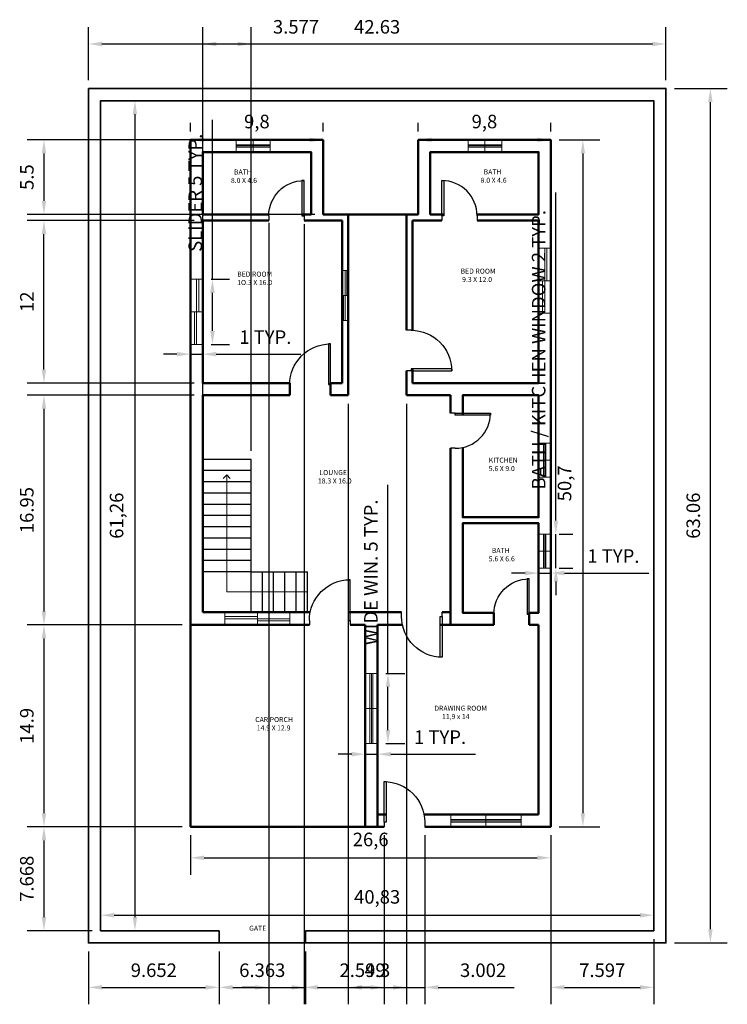
# Model space of a CAD drawing. Units: feet. Extents: x 4235.7 to 4288, y 3917.3 to 3989.9.
import ezdxf

# ---------------------------------------------------------------- set-up
doc = ezdxf.new("R2010")
doc.units = ezdxf.units.FT
for name, color, linetype, lineweight in [('A-ANNO-DIMS', 5, 'Continuous', 18), ('A-ANNO-SYMB', 240, 'Continuous', 18), ('A-ANNO-TEXT', 3, 'Continuous', 30), ('A-AREA-IDEN', 3, 'Continuous', 30), ('A-DOOR', 5, 'Continuous', 25), ('A-FLOR-STRS', 7, 'Continuous', 25), ('A-GLAZ', 2, 'Continuous', 18), ('A-WALL', 7, 'Continuous', 50), ('C-PROP', 242, 'Continuous', 35)]:
    doc.layers.add(name, color=color, linetype=linetype, lineweight=lineweight)
doc.styles.get("Standard").update_dxf_attribs({"font": 'arial.ttf'})
doc.dimstyles.new('ISO-25', dxfattribs={"dimtxt": 1, "dimasz": 1, "dimexe": 1.25, "dimexo": 0.625, "dimtad": 1, "dimtxsty": 'Standard', "dimcen": 1, "dimadec": 0, "dimazin": 0, "dimtfac": 1, "dimtmove": 0, "dimatfit": 3, "dimfxl": 1, "dimarcsym": 0})

# ---------------------------------------------------------------- blocks, each defined once
blk = doc.blocks.new('*U2')
for p, q in [((0, 0), (0, -100)), ((900, 0), (900, -100))]:
    blk.add_line(p, q)
blk.add_lwpolyline([(0, 0), (0, 900), (43.75, 900), (43.75, 0)], close=True)
blk.add_arc((0, 0), 900, 0, 90)
blk = doc.blocks.new('*U3')
for p, q in [((0, 0), (0, -100)), ((750, 0), (750, -100))]:
    blk.add_line(p, q)
blk.add_lwpolyline([(0, 0), (0, 750), (43.75, 750), (43.75, 0)], close=True)
blk.add_arc((0, 0), 750, 0, 90)
blk = doc.blocks.new('*U4')
for p, q in [((0, 0), (0, 100)), ((900, 0), (900, 100))]:
    blk.add_line(p, q)
blk.add_lwpolyline([(0, 0), (0, -900), (43.75, -900), (43.75, 0)], close=True)
blk.add_arc((0, 0), 900, 270, 0)
blk = doc.blocks.new('*U5')
for p, q in [((0, 0), (0, -100)), ((-900, 0), (-900, -100))]:
    blk.add_line(p, q)
blk.add_lwpolyline([(0, 0), (0, 900), (-43.75, 900), (-43.75, 0)], close=True)
blk.add_arc((0, 0), 900, 90, 180)
blk = doc.blocks.new('*D6')
at = {"layer": 'A-ANNO-DIMS', "color": 0, "lineweight": -2, "transparency": 16777216}
for p, q in [((4275.582, 3981.069), (4278.576, 3981.069)), ((4277.326, 3980.069), (4277.326, 3931.369)), ((4275.582, 3930.369), (4278.576, 3930.369))]:
    blk.add_line(p, q, dxfattribs=at)
at = {"layer": 'A-ANNO-DIMS', "color": 0, "transparency": 16777216}
for points in [[(4277.159, 3980.069), (4277.493, 3980.069), (4277.326, 3981.069)], [(4277.159, 3931.369), (4277.493, 3931.369), (4277.326, 3930.369)]]:
    blk.add_solid(points, dxfattribs=at)
at = {"layer": 'Defpoints', "color": 0, "transparency": 16777216}
for p in [(4274.957, 3981.069), (4274.957, 3930.369), (4277.326, 3930.369)]:
    blk.add_point(p, dxfattribs=at)
at = {"layer": 'A-ANNO-DIMS', "color": 0, "transparency": 16777216, "insert": (4276.1, 3955.719), "char_height": 1, "attachment_point": 5, "rotation": 90}
blk.add_mtext('50,7', dxfattribs=at)
blk = doc.blocks.new('*D7')
at = {"layer": 'A-ANNO-DIMS', "color": 0, "lineweight": -2, "transparency": 16777216}
for p, q in [((4248.357, 3981.694), (4248.357, 3982.319)), ((4258.157, 3981.694), (4258.157, 3982.319)), ((4249.357, 3981.069), (4257.157, 3981.069))]:
    blk.add_line(p, q, dxfattribs=at)
at = {"layer": 'A-ANNO-DIMS', "color": 0, "transparency": 16777216}
for points in [[(4249.357, 3981.236), (4249.357, 3980.902), (4248.357, 3981.069)], [(4257.157, 3981.236), (4257.157, 3980.902), (4258.157, 3981.069)]]:
    blk.add_solid(points, dxfattribs=at)
at = {"layer": 'Defpoints', "color": 0, "transparency": 16777216}
for p in [(4248.357, 3981.069), (4258.157, 3981.069), (4258.157, 3981.069)]:
    blk.add_point(p, dxfattribs=at)
at = {"layer": 'A-ANNO-DIMS', "color": 0, "transparency": 16777216, "insert": (4253.257, 3982.295), "char_height": 1, "attachment_point": 5}
blk.add_mtext('9,8', dxfattribs=at)
blk = doc.blocks.new('*D8')
at = {"layer": 'A-ANNO-DIMS', "color": 0, "lineweight": -2, "transparency": 16777216}
for p, q in [((4265.157, 3981.694), (4265.157, 3982.319)), ((4274.957, 3981.694), (4274.957, 3982.319)), ((4266.157, 3981.069), (4273.957, 3981.069))]:
    blk.add_line(p, q, dxfattribs=at)
at = {"layer": 'A-ANNO-DIMS', "color": 0, "transparency": 16777216}
for points in [[(4266.157, 3981.236), (4266.157, 3980.902), (4265.157, 3981.069)], [(4273.957, 3981.236), (4273.957, 3980.902), (4274.957, 3981.069)]]:
    blk.add_solid(points, dxfattribs=at)
at = {"layer": 'Defpoints', "color": 0, "transparency": 16777216}
for p in [(4265.157, 3981.069), (4274.957, 3981.069), (4274.957, 3981.069)]:
    blk.add_point(p, dxfattribs=at)
at = {"layer": 'A-ANNO-DIMS', "color": 0, "transparency": 16777216, "insert": (4270.057, 3982.295), "char_height": 1, "attachment_point": 5}
blk.add_mtext('9,8', dxfattribs=at)
blk = doc.blocks.new('*D9')
at = {"layer": 'A-ANNO-DIMS', "color": 0, "lineweight": -2, "transparency": 16777216}
for p, q in [((4248.357, 3929.744), (4248.357, 3926.829)), ((4274.957, 3929.744), (4274.957, 3926.829)), ((4249.357, 3928.079), (4273.957, 3928.079))]:
    blk.add_line(p, q, dxfattribs=at)
at = {"layer": 'A-ANNO-DIMS', "color": 0, "transparency": 16777216}
for points in [[(4249.357, 3928.245), (4249.357, 3927.912), (4248.357, 3928.079)], [(4273.957, 3928.245), (4273.957, 3927.912), (4274.957, 3928.079)]]:
    blk.add_solid(points, dxfattribs=at)
at = {"layer": 'Defpoints', "color": 0, "transparency": 16777216}
for p in [(4248.357, 3930.369), (4274.957, 3930.369), (4274.957, 3928.079)]:
    blk.add_point(p, dxfattribs=at)
at = {"layer": 'A-ANNO-DIMS', "color": 0, "transparency": 16777216, "insert": (4261.657, 3929.305), "char_height": 1, "attachment_point": 5}
blk.add_mtext('26,6', dxfattribs=at)
blk = doc.blocks.new('*D10')
at = {"layer": 'A-ANNO-DIMS', "color": 0, "lineweight": -2, "transparency": 16777216}
for p, q in [((4241.721, 3923.326), (4241.721, 3925.09)), ((4282.554, 3923.326), (4282.554, 3925.09)), ((4242.721, 3923.84), (4281.554, 3923.84))]:
    blk.add_line(p, q, dxfattribs=at)
at = {"layer": 'A-ANNO-DIMS', "color": 0, "transparency": 16777216}
for points in [[(4242.721, 3924.006), (4242.721, 3923.673), (4241.721, 3923.84)], [(4281.554, 3924.006), (4281.554, 3923.673), (4282.554, 3923.84)]]:
    blk.add_solid(points, dxfattribs=at)
at = {"layer": 'Defpoints', "color": 0, "transparency": 16777216}
for p in [(4282.554, 3923.84), (4241.721, 3922.701), (4282.554, 3922.701)]:
    blk.add_point(p, dxfattribs=at)
at = {"layer": 'A-ANNO-DIMS', "color": 0, "transparency": 16777216, "insert": (4262.137, 3925.066), "char_height": 1, "attachment_point": 5}
blk.add_mtext('40,83', dxfattribs=at)
blk = doc.blocks.new('*D11')
at = {"layer": 'A-ANNO-DIMS', "color": 0, "lineweight": -2, "transparency": 16777216}
for p, q in [((4242.346, 3983.964), (4245.502, 3983.964)), ((4244.252, 3982.964), (4244.252, 3923.701)), ((4242.346, 3922.701), (4245.502, 3922.701))]:
    blk.add_line(p, q, dxfattribs=at)
at = {"layer": 'A-ANNO-DIMS', "color": 0, "transparency": 16777216}
for points in [[(4244.085, 3982.964), (4244.418, 3982.964), (4244.252, 3983.964)], [(4244.085, 3923.701), (4244.418, 3923.701), (4244.252, 3922.701)]]:
    blk.add_solid(points, dxfattribs=at)
at = {"layer": 'Defpoints', "color": 0, "transparency": 16777216}
for p in [(4241.721, 3983.964), (4241.721, 3922.701), (4244.252, 3922.701)]:
    blk.add_point(p, dxfattribs=at)
at = {"layer": 'A-ANNO-DIMS', "color": 0, "transparency": 16777216, "insert": (4243.026, 3953.333), "char_height": 1, "attachment_point": 5, "rotation": 90}
blk.add_mtext('61,26', dxfattribs=at)
blk = doc.blocks.new('WIN-2.496FT')
for p, q in [((0, 2.496), (0.9, 2.496)), ((0.37, 2.496), (0.37, 0)), ((0.45, 2.496), (0.45, 0)), ((0.53, 2.496), (0.53, 0)), ((0.9, 1.248), (0, 1.248)), ((0.45, 1.248), (0.9, 1.248)), ((0, 0), (0.9, 0))]:
    blk.add_line(p, q)
blk = doc.blocks.new('WIN-SLIDER-4.805FT')
for p, q in [((0.45, 0), (0.45, 4.805)), ((0.61, 2.403), (0.61, 4.805)), ((0, 2.403), (0.9, 2.403)), ((0.289, 0), (0.289, 2.403))]:
    blk.add_line(p, q)
for points in [[(0, 4.805), (0.9, 4.805)], [(0.9, 0), (0, 0)]]:
    blk.add_lwpolyline(points)
blk = doc.blocks.new('WIN-5.184FT')
for p, q in [((0, 5.184), (0.9, 5.184)), ((0.35, 5.184), (0.35, 0)), ((0.45, 5.184), (0.45, 0)), ((0.55, 5.184), (0.55, 0)), ((0.9, 2.592), (0, 2.592)), ((0.45, 2.592), (0.9, 2.592)), ((0, 0), (0.9, 0))]:
    blk.add_line(p, q)
blk = doc.blocks.new('*D15')
at = {"layer": 'A-ANNO-DIMS', "color": 0, "lineweight": -2, "transparency": 16777216}
for p, q in [((4275.331, 3952.965), (4275.331, 3977.189)), ((4275.331, 3949.469), (4275.331, 3951.965)), ((4275.582, 3951.965), (4276.581, 3951.965)), ((4275.582, 3949.469), (4276.581, 3949.469)), ((4275.331, 3948.469), (4275.331, 3947.469))]:
    blk.add_line(p, q, dxfattribs=at)
at = {"layer": 'A-ANNO-DIMS', "color": 0, "transparency": 16777216}
for points in [[(4275.165, 3952.965), (4275.498, 3952.965), (4275.331, 3951.965)], [(4275.165, 3948.469), (4275.498, 3948.469), (4275.331, 3949.469)]]:
    blk.add_solid(points, dxfattribs=at)
at = {"layer": 'Defpoints', "color": 0, "transparency": 16777216}
for p in [(4274.957, 3951.965), (4275.331, 3951.965), (4274.957, 3949.469)]:
    blk.add_point(p, dxfattribs=at)
at = {"layer": 'A-ANNO-DIMS', "color": 0, "transparency": 16777216, "insert": (4274.189, 3965.577), "char_height": 1, "attachment_point": 5, "rotation": 90}
blk.add_mtext('BATH / KITCHEN WINDOW 2 TYP.', dxfattribs=at)
blk = doc.blocks.new('*D16')
at = {"layer": 'A-ANNO-DIMS', "color": 0, "lineweight": -2, "transparency": 16777216}
for p, q in [((4273.057, 3949.094), (4272.057, 3949.094)), ((4274.057, 3949.094), (4274.957, 3949.094)), ((4274.057, 3948.844), (4274.057, 3947.844)), ((4274.957, 3948.844), (4274.957, 3947.844)), ((4275.957, 3949.094), (4282.204, 3949.094))]:
    blk.add_line(p, q, dxfattribs=at)
at = {"layer": 'A-ANNO-DIMS', "color": 0, "transparency": 16777216}
for points in [[(4273.057, 3949.261), (4273.057, 3948.928), (4274.057, 3949.094)], [(4275.957, 3949.261), (4275.957, 3948.928), (4274.957, 3949.094)]]:
    blk.add_solid(points, dxfattribs=at)
at = {"layer": 'Defpoints', "color": 0, "transparency": 16777216}
for p in [(4274.057, 3949.469), (4274.957, 3949.469), (4274.957, 3949.094)]:
    blk.add_point(p, dxfattribs=at)
at = {"layer": 'A-ANNO-DIMS', "color": 0, "transparency": 16777216, "insert": (4279.58, 3950.222), "char_height": 1, "attachment_point": 5}
blk.add_mtext('1 TYP.', dxfattribs=at)
blk = doc.blocks.new('*D17')
at = {"layer": 'A-ANNO-DIMS', "color": 0, "lineweight": -2, "transparency": 16777216}
for p, q in [((4249.978, 3970.78), (4249.978, 3982.551)), ((4249.882, 3970.78), (4251.228, 3970.78)), ((4249.978, 3966.975), (4249.978, 3969.78)), ((4249.882, 3965.975), (4251.228, 3965.975))]:
    blk.add_line(p, q, dxfattribs=at)
at = {"layer": 'A-ANNO-DIMS', "color": 0, "transparency": 16777216}
for points in [[(4249.811, 3969.78), (4250.145, 3969.78), (4249.978, 3970.78)], [(4249.811, 3966.975), (4250.145, 3966.975), (4249.978, 3965.975)]]:
    blk.add_solid(points, dxfattribs=at)
at = {"layer": 'Defpoints', "color": 0, "transparency": 16777216}
for p in [(4249.257, 3970.78), (4249.978, 3970.78), (4249.257, 3965.975)]:
    blk.add_point(p, dxfattribs=at)
at = {"layer": 'A-ANNO-DIMS', "color": 0, "transparency": 16777216, "insert": (4248.836, 3977.165), "char_height": 1, "attachment_point": 5, "rotation": 90}
blk.add_mtext('SLIDER 5 TYP.', dxfattribs=at)
blk = doc.blocks.new('*D18')
at = {"layer": 'A-ANNO-DIMS', "color": 0, "lineweight": -2, "transparency": 16777216}
for p, q in [((4247.357, 3965.254), (4246.357, 3965.254)), ((4248.357, 3965.35), (4248.357, 3964.004)), ((4248.357, 3965.254), (4249.257, 3965.254)), ((4249.257, 3965.35), (4249.257, 3964.004)), ((4250.257, 3965.254), (4256.504, 3965.254))]:
    blk.add_line(p, q, dxfattribs=at)
at = {"layer": 'A-ANNO-DIMS', "color": 0, "transparency": 16777216}
for points in [[(4247.357, 3965.421), (4247.357, 3965.088), (4248.357, 3965.254)], [(4250.257, 3965.421), (4250.257, 3965.088), (4249.257, 3965.254)]]:
    blk.add_solid(points, dxfattribs=at)
at = {"layer": 'Defpoints', "color": 0, "transparency": 16777216}
for p in [(4248.357, 3965.975), (4249.257, 3965.975), (4249.257, 3965.254)]:
    blk.add_point(p, dxfattribs=at)
at = {"layer": 'A-ANNO-DIMS', "color": 0, "transparency": 16777216, "insert": (4253.88, 3966.382), "char_height": 1, "attachment_point": 5}
blk.add_mtext('1 TYP.', dxfattribs=at)
blk = doc.blocks.new('*D19')
at = {"layer": 'A-ANNO-DIMS', "color": 0, "lineweight": -2, "transparency": 16777216}
for p, q in [((4262.935, 3941.69), (4262.935, 3955.599)), ((4262.782, 3941.69), (4264.185, 3941.69)), ((4262.935, 3937.506), (4262.935, 3940.69)), ((4262.782, 3936.506), (4264.185, 3936.506))]:
    blk.add_line(p, q, dxfattribs=at)
at = {"layer": 'A-ANNO-DIMS', "color": 0, "transparency": 16777216}
for points in [[(4262.768, 3940.69), (4263.101, 3940.69), (4262.935, 3941.69)], [(4262.768, 3937.506), (4263.101, 3937.506), (4262.935, 3936.506)]]:
    blk.add_solid(points, dxfattribs=at)
at = {"layer": 'Defpoints', "color": 0, "transparency": 16777216}
for p in [(4262.157, 3941.69), (4262.935, 3941.69), (4262.157, 3936.506)]:
    blk.add_point(p, dxfattribs=at)
at = {"layer": 'A-ANNO-DIMS', "color": 0, "transparency": 16777216, "insert": (4261.801, 3949.145), "char_height": 1, "attachment_point": 5, "rotation": 90}
blk.add_mtext('WIDE WIN. 5 TYP.', dxfattribs=at)
blk = doc.blocks.new('*D20')
at = {"layer": 'A-ANNO-DIMS', "color": 0, "lineweight": -2, "transparency": 16777216}
for p, q in [((4260.257, 3935.728), (4259.257, 3935.728)), ((4261.257, 3935.881), (4261.257, 3934.478)), ((4261.257, 3935.728), (4262.157, 3935.728)), ((4262.157, 3935.881), (4262.157, 3934.478)), ((4263.157, 3935.728), (4269.404, 3935.728))]:
    blk.add_line(p, q, dxfattribs=at)
at = {"layer": 'A-ANNO-DIMS', "color": 0, "transparency": 16777216}
for points in [[(4260.257, 3935.895), (4260.257, 3935.561), (4261.257, 3935.728)], [(4263.157, 3935.895), (4263.157, 3935.561), (4262.157, 3935.728)]]:
    blk.add_solid(points, dxfattribs=at)
at = {"layer": 'Defpoints', "color": 0, "transparency": 16777216}
for p in [(4261.257, 3936.506), (4262.157, 3936.506), (4262.157, 3935.728)]:
    blk.add_point(p, dxfattribs=at)
at = {"layer": 'A-ANNO-DIMS', "color": 0, "transparency": 16777216, "insert": (4266.78, 3936.855), "char_height": 1, "attachment_point": 5}
blk.add_mtext('1 TYP.', dxfattribs=at)
blk = doc.blocks.new('*D21')
at = {"layer": 'A-ANNO-DIMS', "color": 0, "lineweight": -2, "transparency": 16777216}
for p, q in [((4240.821, 3985.489), (4240.821, 3989.399)), ((4283.454, 3985.489), (4283.454, 3989.399)), ((4241.821, 3988.149), (4282.454, 3988.149))]:
    blk.add_line(p, q, dxfattribs=at)
at = {"layer": 'A-ANNO-DIMS', "color": 0, "transparency": 16777216}
for points in [[(4241.821, 3988.315), (4241.821, 3987.982), (4240.821, 3988.149)], [(4282.454, 3988.315), (4282.454, 3987.982), (4283.454, 3988.149)]]:
    blk.add_solid(points, dxfattribs=at)
at = {"layer": 'Defpoints', "color": 0, "transparency": 16777216}
for p in [(4283.454, 3988.149), (4240.821, 3984.864), (4283.454, 3984.864)]:
    blk.add_point(p, dxfattribs=at)
at = {"layer": 'A-ANNO-DIMS', "color": 0, "transparency": 16777216, "insert": (4262.137, 3989.285), "char_height": 1, "attachment_point": 5}
blk.add_mtext('42.63', dxfattribs=at)
blk = doc.blocks.new('*D22')
at = {"layer": 'A-ANNO-DIMS', "color": 0, "lineweight": -2, "transparency": 16777216}
for p, q in [((4284.079, 3984.864), (4287.989, 3984.864)), ((4286.739, 3922.801), (4286.739, 3983.864)), ((4284.079, 3921.801), (4287.989, 3921.801))]:
    blk.add_line(p, q, dxfattribs=at)
at = {"layer": 'A-ANNO-DIMS', "color": 0, "transparency": 16777216}
for points in [[(4286.572, 3983.864), (4286.906, 3983.864), (4286.739, 3984.864)], [(4286.572, 3922.801), (4286.906, 3922.801), (4286.739, 3921.801)]]:
    blk.add_solid(points, dxfattribs=at)
at = {"layer": 'Defpoints', "color": 0, "transparency": 16777216}
for p in [(4283.454, 3984.864), (4286.739, 3984.864), (4283.454, 3921.801)]:
    blk.add_point(p, dxfattribs=at)
at = {"layer": 'A-ANNO-DIMS', "color": 0, "transparency": 16777216, "insert": (4285.603, 3953.333), "char_height": 1, "attachment_point": 5, "rotation": 90}
blk.add_mtext('63.06', dxfattribs=at)
blk = doc.blocks.new('*D23')
at = {"layer": 'A-ANNO-DIMS', "color": 0, "lineweight": -2, "transparency": 16777216}
for p, q in [((4250.473, 3921.176), (4250.473, 3917.266)), ((4256.836, 3921.176), (4256.836, 3917.266)), ((4251.473, 3918.516), (4255.836, 3918.516))]:
    blk.add_line(p, q, dxfattribs=at)
at = {"layer": 'A-ANNO-DIMS', "color": 0, "transparency": 16777216}
for points in [[(4251.473, 3918.683), (4251.473, 3918.35), (4250.473, 3918.516)], [(4255.836, 3918.683), (4255.836, 3918.35), (4256.836, 3918.516)]]:
    blk.add_solid(points, dxfattribs=at)
at = {"layer": 'Defpoints', "color": 0, "transparency": 16777216}
for p in [(4250.473, 3921.801), (4256.836, 3921.801), (4256.836, 3918.516)]:
    blk.add_point(p, dxfattribs=at)
at = {"layer": 'A-ANNO-DIMS', "color": 0, "transparency": 16777216, "insert": (4253.654, 3919.652), "char_height": 1, "attachment_point": 5}
blk.add_mtext('6.363', dxfattribs=at)
blk = doc.blocks.new('*D24')
at = {"layer": 'A-ANNO-DIMS', "color": 0, "lineweight": -2, "transparency": 16777216}
for p, q in [((4240.821, 3921.176), (4240.821, 3917.266)), ((4250.473, 3921.176), (4250.473, 3917.266)), ((4241.821, 3918.516), (4249.473, 3918.516))]:
    blk.add_line(p, q, dxfattribs=at)
at = {"layer": 'A-ANNO-DIMS', "color": 0, "transparency": 16777216}
for points in [[(4241.821, 3918.683), (4241.821, 3918.35), (4240.821, 3918.516)], [(4249.473, 3918.683), (4249.473, 3918.35), (4250.473, 3918.516)]]:
    blk.add_solid(points, dxfattribs=at)
at = {"layer": 'Defpoints', "color": 0, "transparency": 16777216}
for p in [(4240.821, 3921.801), (4250.473, 3921.801), (4250.473, 3918.516)]:
    blk.add_point(p, dxfattribs=at)
at = {"layer": 'A-ANNO-DIMS', "color": 0, "transparency": 16777216, "insert": (4245.647, 3919.652), "char_height": 1, "attachment_point": 5}
blk.add_mtext('9.652', dxfattribs=at)
blk = doc.blocks.new('*D25')
at = {"layer": 'A-ANNO-DIMS', "color": 0, "lineweight": -2, "transparency": 16777216}
for p, q in [((4274.957, 3929.744), (4274.957, 3917.266)), ((4282.554, 3922.076), (4282.554, 3917.266)), ((4275.957, 3918.516), (4281.554, 3918.516))]:
    blk.add_line(p, q, dxfattribs=at)
at = {"layer": 'A-ANNO-DIMS', "color": 0, "transparency": 16777216}
for points in [[(4275.957, 3918.683), (4275.957, 3918.35), (4274.957, 3918.516)], [(4281.554, 3918.683), (4281.554, 3918.35), (4282.554, 3918.516)]]:
    blk.add_solid(points, dxfattribs=at)
at = {"layer": 'Defpoints', "color": 0, "transparency": 16777216}
for p in [(4274.957, 3930.369), (4282.554, 3922.701), (4282.554, 3918.516)]:
    blk.add_point(p, dxfattribs=at)
at = {"layer": 'A-ANNO-DIMS', "color": 0, "transparency": 16777216, "insert": (4278.756, 3919.652), "char_height": 1, "attachment_point": 5}
blk.add_mtext('7.597', dxfattribs=at)
blk = doc.blocks.new('*D26')
at = {"layer": 'A-ANNO-DIMS', "color": 0, "lineweight": -2, "transparency": 16777216}
for p, q in [((4247.732, 3930.369), (4236.286, 3930.369)), ((4237.536, 3929.369), (4237.536, 3923.701)), ((4241.096, 3922.701), (4236.286, 3922.701))]:
    blk.add_line(p, q, dxfattribs=at)
at = {"layer": 'A-ANNO-DIMS', "color": 0, "transparency": 16777216}
for points in [[(4237.369, 3929.369), (4237.702, 3929.369), (4237.536, 3930.369)], [(4237.369, 3923.701), (4237.702, 3923.701), (4237.536, 3922.701)]]:
    blk.add_solid(points, dxfattribs=at)
at = {"layer": 'Defpoints', "color": 0, "transparency": 16777216}
for p in [(4248.357, 3930.369), (4237.536, 3922.701), (4241.721, 3922.701)]:
    blk.add_point(p, dxfattribs=at)
at = {"layer": 'A-ANNO-DIMS', "color": 0, "transparency": 16777216, "insert": (4236.4, 3926.535), "char_height": 1, "attachment_point": 5, "rotation": 90}
blk.add_mtext('7.668', dxfattribs=at)
blk = doc.blocks.new('*D27')
at = {"layer": 'A-ANNO-DIMS', "color": 0, "lineweight": -2, "transparency": 16777216}
for p, q in [((4247.732, 3945.269), (4236.286, 3945.269)), ((4237.536, 3944.269), (4237.536, 3931.369)), ((4247.732, 3930.369), (4236.286, 3930.369))]:
    blk.add_line(p, q, dxfattribs=at)
at = {"layer": 'A-ANNO-DIMS', "color": 0, "transparency": 16777216}
for points in [[(4237.369, 3944.269), (4237.702, 3944.269), (4237.536, 3945.269)], [(4237.369, 3931.369), (4237.702, 3931.369), (4237.536, 3930.369)]]:
    blk.add_solid(points, dxfattribs=at)
at = {"layer": 'Defpoints', "color": 0, "transparency": 16777216}
for p in [(4248.357, 3945.269), (4237.536, 3930.369), (4248.357, 3930.369)]:
    blk.add_point(p, dxfattribs=at)
at = {"layer": 'A-ANNO-DIMS', "color": 0, "transparency": 16777216, "insert": (4236.4, 3937.819), "char_height": 1, "attachment_point": 5, "rotation": 90}
blk.add_mtext('14.9', dxfattribs=at)
blk = doc.blocks.new('*D28')
at = {"layer": 'A-ANNO-DIMS', "color": 0, "lineweight": -2, "transparency": 16777216}
for p, q in [((4248.632, 3962.219), (4236.286, 3962.219)), ((4237.536, 3961.219), (4237.536, 3946.269)), ((4247.732, 3945.269), (4236.286, 3945.269))]:
    blk.add_line(p, q, dxfattribs=at)
at = {"layer": 'A-ANNO-DIMS', "color": 0, "transparency": 16777216}
for points in [[(4237.369, 3961.219), (4237.702, 3961.219), (4237.536, 3962.219)], [(4237.369, 3946.269), (4237.702, 3946.269), (4237.536, 3945.269)]]:
    blk.add_solid(points, dxfattribs=at)
at = {"layer": 'Defpoints', "color": 0, "transparency": 16777216}
for p in [(4249.257, 3962.219), (4237.536, 3945.269), (4248.357, 3945.269)]:
    blk.add_point(p, dxfattribs=at)
at = {"layer": 'A-ANNO-DIMS', "color": 0, "transparency": 16777216, "insert": (4236.4, 3953.744), "char_height": 1, "attachment_point": 5, "rotation": 90}
blk.add_mtext('16.95', dxfattribs=at)
blk = doc.blocks.new('*D29')
at = {"layer": 'A-ANNO-DIMS', "color": 0, "lineweight": -2, "transparency": 16777216}
for p, q in [((4248.632, 3975.119), (4236.286, 3975.119)), ((4237.536, 3964.119), (4237.536, 3974.119)), ((4248.632, 3963.119), (4236.286, 3963.119))]:
    blk.add_line(p, q, dxfattribs=at)
at = {"layer": 'A-ANNO-DIMS', "color": 0, "transparency": 16777216}
for points in [[(4237.369, 3974.119), (4237.702, 3974.119), (4237.536, 3975.119)], [(4237.369, 3964.119), (4237.702, 3964.119), (4237.536, 3963.119)]]:
    blk.add_solid(points, dxfattribs=at)
at = {"layer": 'Defpoints', "color": 0, "transparency": 16777216}
for p in [(4237.536, 3975.119), (4249.257, 3975.119), (4249.257, 3963.119)]:
    blk.add_point(p, dxfattribs=at)
at = {"layer": 'A-ANNO-DIMS', "color": 0, "transparency": 16777216, "insert": (4236.409, 3969.119), "char_height": 1, "attachment_point": 5, "rotation": 90}
blk.add_mtext('12', dxfattribs=at)
blk = doc.blocks.new('*D30')
at = {"layer": 'A-ANNO-DIMS', "color": 0, "lineweight": -2, "transparency": 16777216}
for p, q in [((4257.532, 3981.069), (4236.286, 3981.069)), ((4237.536, 3980.069), (4237.536, 3976.569)), ((4257.532, 3975.569), (4236.286, 3975.569))]:
    blk.add_line(p, q, dxfattribs=at)
at = {"layer": 'A-ANNO-DIMS', "color": 0, "transparency": 16777216}
for points in [[(4237.369, 3980.069), (4237.702, 3980.069), (4237.536, 3981.069)], [(4237.369, 3976.569), (4237.702, 3976.569), (4237.536, 3975.569)]]:
    blk.add_solid(points, dxfattribs=at)
at = {"layer": 'Defpoints', "color": 0, "transparency": 16777216}
for p in [(4258.157, 3981.069), (4237.536, 3975.569), (4258.157, 3975.569)]:
    blk.add_point(p, dxfattribs=at)
at = {"layer": 'A-ANNO-DIMS', "color": 0, "transparency": 16777216, "insert": (4236.402, 3978.319), "char_height": 1, "attachment_point": 5, "rotation": 90}
blk.add_mtext('5.5', dxfattribs=at)
blk = doc.blocks.new('*D31')
at = {"layer": 'A-ANNO-DIMS', "color": 0, "lineweight": -2, "transparency": 16777216}
for p, q in [((4249.257, 3958.111), (4249.257, 3989.399)), ((4252.834, 3958.111), (4252.834, 3989.399)), ((4250.257, 3988.149), (4251.834, 3988.149)), ((4252.834, 3988.149), (4258.458, 3988.149))]:
    blk.add_line(p, q, dxfattribs=at)
at = {"layer": 'A-ANNO-DIMS', "color": 0, "transparency": 16777216}
for points in [[(4250.257, 3988.315), (4250.257, 3987.982), (4249.257, 3988.149)], [(4251.834, 3988.315), (4251.834, 3987.982), (4252.834, 3988.149)]]:
    blk.add_solid(points, dxfattribs=at)
at = {"layer": 'Defpoints', "color": 0, "transparency": 16777216}
for p in [(4252.834, 3988.149), (4249.257, 3957.486), (4252.834, 3957.486)]:
    blk.add_point(p, dxfattribs=at)
at = {"layer": 'A-ANNO-DIMS', "color": 0, "transparency": 16777216, "insert": (4256.146, 3989.285), "char_height": 1, "attachment_point": 5}
blk.add_mtext('3.577', dxfattribs=at)
blk = doc.blocks.new('*D32')
at = {"layer": 'A-ANNO-DIMS', "color": 0, "lineweight": -2, "transparency": 16777216}
for p, q in [((4260.007, 3961.594), (4260.007, 3917.266)), ((4264.307, 3961.594), (4264.307, 3917.266)), ((4261.007, 3918.516), (4263.307, 3918.516))]:
    blk.add_line(p, q, dxfattribs=at)
at = {"layer": 'A-ANNO-DIMS', "color": 0, "transparency": 16777216}
for points in [[(4261.007, 3918.683), (4261.007, 3918.35), (4260.007, 3918.516)], [(4263.307, 3918.683), (4263.307, 3918.35), (4264.307, 3918.516)]]:
    blk.add_solid(points, dxfattribs=at)
at = {"layer": 'Defpoints', "color": 0, "transparency": 16777216}
for p in [(4260.007, 3962.219), (4264.307, 3962.219), (4264.307, 3918.516)]:
    blk.add_point(p, dxfattribs=at)
at = {"layer": 'A-ANNO-DIMS', "color": 0, "transparency": 16777216, "insert": (4262.157, 3919.652), "char_height": 1, "attachment_point": 5}
blk.add_mtext('4.3', dxfattribs=at)
blk = doc.blocks.new('*D33')
at = {"layer": 'A-ANNO-DIMS', "color": 0, "lineweight": -2, "transparency": 16777216}
for p, q in [((4254.138, 3974.944), (4254.138, 3917.266)), ((4256.737, 3974.841), (4256.737, 3917.266)), ((4253.138, 3918.516), (4252.138, 3918.516)), ((4254.138, 3918.516), (4256.737, 3918.516)), ((4257.737, 3918.516), (4263.381, 3918.516))]:
    blk.add_line(p, q, dxfattribs=at)
at = {"layer": 'A-ANNO-DIMS', "color": 0, "transparency": 16777216}
for points in [[(4253.138, 3918.683), (4253.138, 3918.35), (4254.138, 3918.516)], [(4257.737, 3918.683), (4257.737, 3918.35), (4256.737, 3918.516)]]:
    blk.add_solid(points, dxfattribs=at)
at = {"layer": 'Defpoints', "color": 0, "transparency": 16777216}
for p in [(4254.138, 3975.569), (4256.737, 3975.466), (4256.737, 3918.516)]:
    blk.add_point(p, dxfattribs=at)
at = {"layer": 'A-ANNO-DIMS', "color": 0, "transparency": 16777216, "insert": (4261.059, 3919.652), "char_height": 1, "attachment_point": 5}
blk.add_mtext('2.599', dxfattribs=at)
blk = doc.blocks.new('*D34')
at = {"layer": 'A-ANNO-DIMS', "color": 0, "lineweight": -2, "transparency": 16777216}
for p, q in [((4262.649, 3929.744), (4262.649, 3917.266)), ((4265.651, 3929.744), (4265.651, 3917.266)), ((4261.649, 3918.516), (4260.649, 3918.516)), ((4262.649, 3918.516), (4265.651, 3918.516)), ((4266.651, 3918.516), (4272.264, 3918.516))]:
    blk.add_line(p, q, dxfattribs=at)
at = {"layer": 'A-ANNO-DIMS', "color": 0, "transparency": 16777216}
for points in [[(4261.649, 3918.683), (4261.649, 3918.35), (4262.649, 3918.516)], [(4266.651, 3918.683), (4266.651, 3918.35), (4265.651, 3918.516)]]:
    blk.add_solid(points, dxfattribs=at)
at = {"layer": 'Defpoints', "color": 0, "transparency": 16777216}
for p in [(4262.649, 3930.369), (4265.651, 3930.369), (4265.651, 3918.516)]:
    blk.add_point(p, dxfattribs=at)
at = {"layer": 'A-ANNO-DIMS', "color": 0, "transparency": 16777216, "insert": (4269.957, 3919.652), "char_height": 1, "attachment_point": 5}
blk.add_mtext('3.002', dxfattribs=at)

msp = doc.modelspace()

# ---------------------------------------------------------------- linework, layer by layer
at = {"layer": 'A-ANNO-SYMB'}
for p, q in [((4251.0457, 3956.3391), (4250.7651, 3956.0748)), ((4251.0457, 3947.7023), (4251.0457, 3956.3391)), ((4251.0457, 3956.3391), (4251.2945, 3956.0748)), ((4256.9843, 3947.7023), (4251.0457, 3947.7023))]:
    msp.add_line(p, q, dxfattribs=at)
at = {"layer": 'A-FLOR-STRS'}
for p, q in [((4252.8343, 3957.4857), (4249.2571, 3957.4857)), ((4252.8343, 3949.1857), (4252.8343, 3957.4857)), ((4252.8343, 3956.6557), (4249.2571, 3956.6557)), ((4252.8343, 3955.8257), (4249.2571, 3955.8257)), ((4252.8343, 3954.9957), (4249.2571, 3954.9957)), ((4252.8343, 3954.1657), (4249.2571, 3954.1657)), ((4252.8343, 3953.3357), (4249.2571, 3953.3357)), ((4252.8343, 3952.5057), (4249.2571, 3952.5057)), ((4252.8343, 3951.6757), (4249.2571, 3951.6757)), ((4252.8343, 3950.8457), (4249.2571, 3950.8457)), ((4252.8343, 3950.0157), (4249.2571, 3950.0157)), ((4252.8343, 3949.1857), (4249.2571, 3949.1857)), ((4249.2571, 3949.1857), (4249.2571, 3946.2188)), ((4252.8343, 3949.1857), (4256.9843, 3949.1857)), ((4252.8343, 3946.2188), (4252.8343, 3949.1857)), ((4253.6643, 3946.2188), (4253.6643, 3949.1857)), ((4254.4943, 3946.2188), (4254.4943, 3949.1857)), ((4255.3243, 3946.2188), (4255.3243, 3949.1857)), ((4256.1543, 3946.2188), (4256.1543, 3949.1857)), ((4256.9843, 3946.2188), (4256.9843, 3949.1857)), ((4249.2571, 3946.2188), (4252.8343, 3946.2188))]:
    msp.add_line(p, q, dxfattribs=at)
at = {"layer": 'A-GLAZ'}
for p, q in [((4259.7657, 3967.7439), (4259.7657, 3971.4232)), ((4259.8883, 3969.5836), (4259.8883, 3971.4232)), ((4259.5571, 3969.5836), (4260.0071, 3969.5836)), ((4259.643, 3967.7439), (4259.643, 3969.5836))]:
    msp.add_line(p, q, dxfattribs=at)
for points in [[(4259.5571, 3971.4232), (4260.0071, 3971.4232)], [(4260.0071, 3967.7439), (4259.5571, 3967.7439)]]:
    msp.add_lwpolyline(points, dxfattribs=at)
at = {"layer": 'A-WALL'}
for p, q in [((4260.0071, 3975.5688), (4260.0071, 3962.2188)), ((4264.3071, 3975.5688), (4264.3071, 3967.016)), ((4249.2571, 3975.1188), (4254.1362, 3975.1188)), ((4249.2571, 3963.1188), (4249.2571, 3975.1188)), ((4256.7374, 3975.1188), (4259.5571, 3975.1188)), ((4259.5571, 3975.1188), (4259.5571, 3963.1188)), ((4264.7571, 3975.1188), (4264.7571, 3967.0137)), ((4266.9119, 3975.1188), (4264.7571, 3975.1188)), ((4274.0571, 3975.1188), (4269.5131, 3975.1188)), ((4274.0571, 3963.1188), (4274.0571, 3975.1188)), ((4264.3071, 3964.0143), (4264.3071, 3962.2188)), ((4264.7571, 3964.1602), (4264.7571, 3963.1188)), ((4255.6832, 3963.1188), (4249.2571, 3963.1188)), ((4255.6832, 3963.1188), (4255.6832, 3962.2188)), ((4259.5571, 3963.1188), (4258.6832, 3963.1188)), ((4258.6832, 3963.1188), (4258.6832, 3962.2188)), ((4264.7571, 3963.1188), (4274.0571, 3963.1188)), ((4249.2571, 3962.2188), (4255.6832, 3962.2188)), ((4249.2571, 3946.2188), (4249.2571, 3962.2188)), ((4258.6832, 3962.2188), (4260.0071, 3962.2188)), ((4264.3071, 3962.2188), (4267.5571, 3962.2188)), ((4267.5571, 3962.2188), (4267.5571, 3960.9051)), ((4267.5571, 3958.3039), (4267.5571, 3946.2188)), ((4257.1982, 3946.2188), (4249.2571, 3946.2188)), ((4263.9442, 3946.2188), (4259.99, 3946.2188)), ((4267.5571, 3946.2188), (4266.9459, 3946.2188)), ((4267.5571, 3946.2188), (4267.5571, 3945.2688)), ((4270.7549, 3946.1688), (4270.7549, 3945.2688)), ((4273.3549, 3946.1688), (4273.3549, 3945.2688)), ((4257.1342, 3945.2688), (4248.3571, 3945.2688)), ((4261.2571, 3945.2688), (4260.1359, 3945.2688)), ((4261.2571, 3945.2688), (4261.2571, 3930.3688)), ((4262.1571, 3945.2688), (4262.1571, 3931.2688)), ((4264.0082, 3945.2688), (4262.1571, 3945.2688)), ((4270.7549, 3945.2688), (4266.8, 3945.2688)), ((4274.0571, 3945.2688), (4273.3549, 3945.2688)), ((4274.0571, 3931.2688), (4274.0571, 3945.2688)), ((4262.1571, 3931.2688), (4262.7948, 3931.2688)), ((4262.1571, 3931.2688), (4262.1571, 3930.3688)), ((4265.5967, 3931.2688), (4274.0571, 3931.2688))]:
    msp.add_line(p, q, dxfattribs=at)
for points in [[(4262.6489, 3930.3688), (4248.3571, 3930.3688), (4248.3571, 3946.2188), (4248.3571, 3963.1188), (4248.3571, 3981.0688), (4258.1571, 3981.0688)], [(4258.1571, 3981.0688), (4258.1571, 3975.5688), (4265.1571, 3975.5688), (4265.1571, 3981.0688)], [(4265.1571, 3981.0688), (4274.9571, 3981.0688), (4274.9571, 3930.3688), (4265.6506, 3930.3688)], [(4254.1382, 3975.5688), (4249.2571, 3975.5688), (4249.2571, 3980.1688), (4257.2571, 3980.1688), (4257.2571, 3975.5688), (4256.5857, 3975.5688)], [(4269.5111, 3975.5688), (4274.0571, 3975.5688), (4274.0571, 3980.1688), (4266.0571, 3980.1688), (4266.0571, 3975.5688), (4267.0637, 3975.5688)], [(4268.4571, 3958.3634), (4268.4571, 3953.2188), (4274.0571, 3953.2188), (4274.0571, 3962.2188), (4268.4571, 3962.2188), (4268.4571, 3960.7534)], [(4273.3549, 3946.1688), (4274.0571, 3946.1688), (4274.0571, 3952.7688), (4268.4571, 3952.7688), (4268.4571, 3946.1688), (4270.7549, 3946.1688)]]:
    msp.add_lwpolyline(points, dxfattribs=at)
at = {"layer": 'C-PROP'}
for p, q in [((4250.4728, 3922.7012), (4250.4728, 3921.8012)), ((4256.8358, 3922.7012), (4256.8358, 3921.8012))]:
    msp.add_line(p, q, dxfattribs=at)
msp.add_lwpolyline([(4240.8207, 3984.8638), (4283.4541, 3984.8638), (4283.4541, 3921.8012), (4240.8207, 3921.8012)], close=True, dxfattribs=at)
msp.add_lwpolyline([(4250.4728, 3922.7012), (4241.7207, 3922.7012), (4241.7207, 3983.9638), (4282.5541, 3983.9638), (4282.5541, 3922.7012), (4256.8358, 3922.7012)], dxfattribs=at)

# ---------------------------------------------------------------- block references
at = {"layer": 'A-DOOR'}
for name, p, xscale, yscale, zscale in [('*U3', (4256.7374, 3975.4657), -0.0034682910877258, 0.0034682910877258, 0.0034682910877258), ('*U3', (4266.9119, 3975.4657), 0.0034682910877258, 0.0034682910877258, 0.0034682910877258), ('*U2', (4258.6832, 3963.0024), -0.0033352546469728, 0.0033352546469728, 0.0033352546469728), ('*U2', (4260.1359, 3945.6024), -0.0033352546469728, 0.0033352546469728, 0.0033352546469728), ('*U3', (4273.3549, 3946.0657), -0.0034682910877258, 0.0034682910877258, 0.0034682910877258), ('*U4', (4266.9459, 3945.8853), -0.0033352546469728, 0.0033352546469728, 0.0033352546469728), ('*U5', (4262.6489, 3930.7024), -0.0033352546469728, 0.0033352546469728, 0.0033352546469728)]:
    msp.add_blockref(name, p, dxfattribs=dict(at, xscale=xscale, yscale=yscale, zscale=zscale))
at = {"layer": 'A-DOOR', "rotation": 270}
for name, p, xscale, yscale, zscale in [('*U2', (4264.6406, 3964.0143), -0.0033352546469728, 0.0033352546469728, 0.0033352546469728), ('*U3', (4267.9039, 3960.9051), 0.0034682910877258, 0.0034682910877258, 0.0034682910877258)]:
    msp.add_blockref(name, p, dxfattribs=dict(at, xscale=xscale, yscale=yscale, zscale=zscale))
at = {"layer": 'A-GLAZ'}
for name, p, rotation in [('WIN-2.496FT', (4254.23, 3980.1688), 90.0000000000252), ('WIN-2.496FT', (4271.3453, 3980.1688), 90.0000000000252), ('WIN-SLIDER-4.805FT', (4250.8928, 3946.1689), 270), ('WIN-5.184FT', (4267.5781, 3931.2689), 270.0000000000054)]:
    msp.add_blockref(name, p, dxfattribs=dict(at, rotation=rotation))
for name, p in [('WIN-SLIDER-4.805FT', (4274.057, 3968.2739)), ('WIN-SLIDER-4.805FT', (4248.357, 3965.975)), ('WIN-2.496FT', (4274.057, 3956.178)), ('WIN-2.496FT', (4274.057, 3949.469)), ('WIN-5.184FT', (4261.257, 3936.506))]:
    msp.add_blockref(name, p, dxfattribs=at)

# ---------------------------------------------------------------- texts
at = {"layer": 'A-ANNO-TEXT', "insert": (4252.6883, 3923.0639), "char_height": 0.37161, "attachment_point": 1}
msp.add_mtext_dynamic_manual_height_columns('\\pxt0;GATE ', width=11.300658, gutter_width=83.2236, heights=[11.4847], dxfattribs=at)
at = {"layer": 'A-AREA-IDEN', "char_height": 0.37161, "attachment_point": 1}
for s, width, gutter_width, heights, insert in [('\\pxt0;  BATH\\P8.0 X 4.6', 11.300658, 83.2236, [11.4847], (4251.3384, 3978.8836)), ('\\pxt0;  BATH\\P8.0 X 4.6', 11.300658, 83.2236, [11.4847], (4269.7726, 3978.8929)), ('\\pxt0;  BED ROOM\\P  1O.3 X 16.0', 11.300658, 83.2236, [11.4847], (4251.5753, 3971.3475)), ('\\pxt0;  BED ROOM\\P   9.3 X 12.0', 11.300658, 83.2236, [11.4847], (4268.0698, 3971.57)), ('\\pxt0;KITCHEN\\P5.6 X 9.0', 11.300658, 83.2236, [11.4847], (4270.3752, 3957.6145)), ('\\pxt0; LOUNGE\\P18.3 X 16.0', 11.300658, 83.2236, [11.4847], (4257.7608, 3956.7017)), ('\\pxt0;  BATH\\P5.6 X 6.6', 11.300658, 83.2236, [11.4847], (4270.3752, 3950.9531)), ('\\pxt0;DRAWING ROOM\\P     11,9 x 14', 6.307461, 46.4512, [6.4102], (4266.3568, 3939.3061)), ('\\pxt0;CAR PORCH\\P 14.9 X 12.9 ', 11.300658, 83.2236, [11.4847], (4253.1351, 3938.4712))]:
    msp.add_mtext_dynamic_manual_height_columns(s, width=width, gutter_width=gutter_width, heights=heights, dxfattribs=dict(at, insert=insert))

# ---------------------------------------------------------------- dimensions: what is measured, and where the dimension line sits
at = {"layer": 'A-ANNO-DIMS'}
for base, p1, p2, override, picture, middle in [((4283.4541, 3988.1488), (4240.8207, 3984.8638), (4283.4541, 3984.8638), {"dimdec": 2, "dimlfac": 1, "dimrnd": 0, "dimzin": 0, "dimdsep": 46, "dimlunit": 2}, '*D21', (4262.1374, 3989.2847)), ((4252.8343, 3988.1488), (4249.2571, 3957.4857), (4252.8343, 3957.4857), {"dimdec": 3, "dimlfac": 1, "dimrnd": 0, "dimzin": 0, "dimdsep": 46, "dimlunit": 2}, '*D31', (4256.1462, 3989.2847)), ((4258.1571, 3981.0688), (4248.3571, 3981.0688), (4258.1571, 3981.0688), {"dimclrd": 0, "dimclre": 0, "dimclrt": 0}, '*D7', (4253.2571, 3982.2948)), ((4274.9571, 3981.0688), (4265.1571, 3981.0688), (4274.9571, 3981.0688), {"dimclrd": 0, "dimclre": 0, "dimclrt": 0}, '*D8', (4270.0571, 3982.2948)), ((4256.7374, 3918.5162), (4254.1382, 3975.5688), (4256.7374, 3975.4657), {"dimdec": 3, "dimlfac": 1, "dimrnd": 0, "dimzin": 0, "dimdsep": 46, "dimlunit": 2}, '*D33', (4261.0592, 3919.6518)), ((4264.3071, 3918.5162), (4260.0071, 3962.2188), (4264.3071, 3962.2188), {"dimdec": 1, "dimlfac": 1, "dimrnd": 0, "dimzin": 0, "dimdsep": 46, "dimlunit": 2}, '*D32', (4262.1571, 3919.6521)), ((4274.9571, 3928.0788), (4248.3571, 3930.3688), (4274.9571, 3930.3688), {"dimclrd": 0, "dimclre": 0, "dimclrt": 0}, '*D9', (4261.6571, 3929.3047)), ((4265.6506, 3918.5162), (4262.6489, 3930.3688), (4265.6506, 3930.3688), {"dimdec": 3, "dimlfac": 1, "dimrnd": 0, "dimzin": 0, "dimdsep": 46, "dimlunit": 2}, '*D34', (4269.9574, 3919.6521)), ((4282.5541, 3918.5162), (4274.9571, 3930.3688), (4282.5541, 3922.7012), {"dimdec": 3, "dimlfac": 1, "dimrnd": 0, "dimzin": 0, "dimdsep": 46, "dimlunit": 2}, '*D25', (4278.7556, 3919.6518)), ((4282.5541, 3923.8397), (4241.7207, 3922.7012), (4282.5541, 3922.7012), {"dimclrd": 0, "dimclre": 0, "dimclrt": 0}, '*D10', (4262.1374, 3925.0656)), ((4250.4728, 3918.5162), (4240.8207, 3921.8012), (4250.4728, 3921.8012), {"dimdec": 3, "dimlfac": 1, "dimrnd": 0, "dimzin": 0, "dimdsep": 46, "dimlunit": 2}, '*D24', (4245.6468, 3919.6518)), ((4256.8358, 3918.5162), (4250.4728, 3921.8012), (4256.8358, 3921.8012), {"dimdec": 3, "dimlfac": 1, "dimrnd": 0, "dimzin": 0, "dimdsep": 46, "dimlunit": 2}, '*D23', (4253.6543, 3919.6521))]:
    dim = msp.add_linear_dim(base=base, p1=p1, p2=p2, dimstyle='ISO-25', override=override, dxfattribs=at)
    dim.commit()
    dim.dimension.update_dxf_attribs({"geometry": picture, "text_midpoint": middle})
for base, p1, p2, override, picture, middle in [((4286.7391, 3984.8638), (4283.4541, 3921.8012), (4283.4541, 3984.8638), {"dimdec": 2, "dimlfac": 1, "dimrnd": 0, "dimzin": 0, "dimdsep": 46, "dimlunit": 2}, '*D22', (4285.6032, 3953.3325)), ((4237.5357, 3975.5688), (4258.1571, 3981.0688), (4258.1571, 3975.5688), {"dimdec": 1, "dimlfac": 1, "dimrnd": 0, "dimzin": 0, "dimdsep": 46, "dimlunit": 2}, '*D30', (4236.4022, 3978.3188)), ((4237.5357, 3975.1188), (4249.2571, 3963.1188), (4249.2571, 3975.1188), {"dimdec": 0, "dimlfac": 1, "dimrnd": 0, "dimzin": 0, "dimdsep": 46, "dimlunit": 2}, '*D29', (4236.4087, 3969.1188)), ((4237.5357, 3945.2688), (4249.2571, 3962.2188), (4248.3571, 3945.2688), {"dimdec": 2, "dimlfac": 1, "dimrnd": 0, "dimzin": 0, "dimdsep": 46, "dimlunit": 2}, '*D28', (4236.4002, 3953.7438)), ((4237.5357, 3930.3688), (4248.3571, 3945.2688), (4248.3571, 3930.3688), {"dimdec": 1, "dimlfac": 1, "dimrnd": 0, "dimzin": 0, "dimdsep": 46, "dimlunit": 2}, '*D27', (4236.4002, 3937.8188)), ((4237.5357, 3922.7012), (4248.3571, 3930.3688), (4241.7207, 3922.7012), {"dimdec": 3, "dimlfac": 1, "dimrnd": 0, "dimzin": 0, "dimdsep": 46, "dimlunit": 2}, '*D26', (4236.4002, 3926.535))]:
    dim = msp.add_linear_dim(base=base, p1=p1, p2=p2, angle=90, dimstyle='ISO-25', override=override, dxfattribs=at)
    dim.commit()
    dim.dimension.update_dxf_attribs({"geometry": picture, "text_midpoint": middle})
for base, p1, p2, picture, middle in [((4244.2518, 3922.7012), (4241.7207, 3983.9638), (4241.7207, 3922.7012), '*D11', (4244.2518, 3953.3325)), ((4277.3259, 3930.3688), (4274.9571, 3981.0688), (4274.9571, 3930.3688), '*D6', (4277.3259, 3955.7188))]:
    dim = msp.add_linear_dim(base=base, p1=p1, p2=p2, angle=90, dimstyle='ISO-25', override={"dimclrd": 0, "dimclre": 0, "dimclrt": 0}, dxfattribs=at)
    dim.commit()
    dim.dimension.update_dxf_attribs({"geometry": picture, "text_midpoint": middle, "dimtype": 160})
for base, p1, p2, text, picture, middle in [((4249.9778, 3970.7801), (4249.2571, 3965.975), (4249.2571, 3970.7801), 'SLIDER <> TYP.', '*D17', (4248.8358, 3977.1653)), ((4275.3315, 3951.965), (4274.9571, 3949.4688), (4274.9571, 3951.965), 'BATH / KITCHEN WINDOW <> TYP.', '*D15', (4274.1891, 3965.577)), ((4262.9348, 3941.6904), (4262.1571, 3936.5057), (4262.1571, 3941.6904), 'WIDE WIN. <> TYP.', '*D19', (4261.8013, 3949.1448))]:
    dim = msp.add_linear_dim(base=base, p1=p1, p2=p2, angle=90, text=text, dimstyle='ISO-25', override={"dimdec": 0, "dimlfac": 1, "dimrnd": 0, "dimzin": 0, "dimdsep": 46, "dimlunit": 2}, dxfattribs=at)
    dim.commit()
    dim.dimension.update_dxf_attribs({"geometry": picture, "text_midpoint": middle})
for base, p1, p2, picture, middle in [((4249.2571, 3965.2542), (4248.3571, 3965.975), (4249.2571, 3965.975), '*D18', (4253.8804, 3966.3816)), ((4274.9571, 3949.0944), (4274.0571, 3949.4688), (4274.9571, 3949.4688), '*D16', (4279.5804, 3950.2218)), ((4262.1571, 3935.728), (4261.2571, 3936.5057), (4262.1571, 3936.5057), '*D20', (4266.7804, 3936.8554))]:
    dim = msp.add_linear_dim(base=base, p1=p1, p2=p2, text='<> TYP.', dimstyle='ISO-25', override={"dimdec": 0, "dimlfac": 1, "dimrnd": 0, "dimzin": 0, "dimdsep": 46, "dimlunit": 2}, dxfattribs=at)
    dim.commit()
    dim.dimension.update_dxf_attribs({"geometry": picture, "text_midpoint": middle})

doc.saveas('drawing.dxf')
